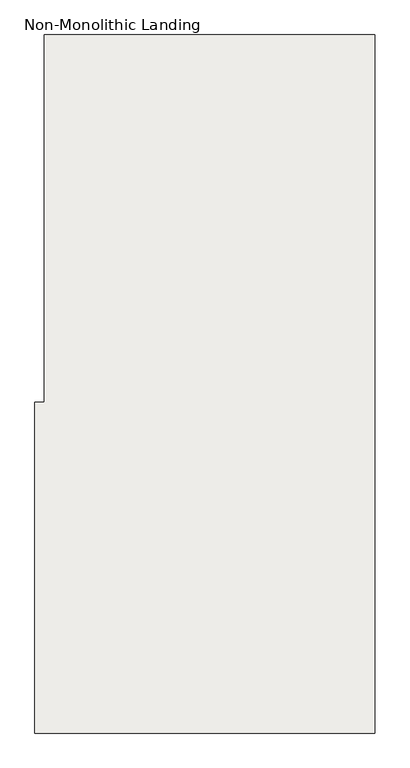
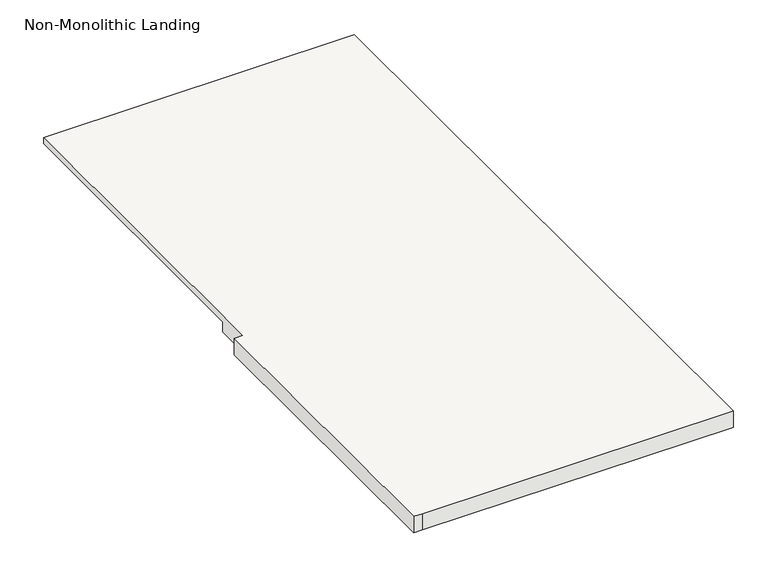
"""IFC4 building model written with IfcOpenShell, lengths in millimetres: slab geometry, Non-Monolithic Landing."""

from ifc_helpers import new_model, si_unit, origin, place, context, project, spatial, faceted_brep, source, transform, mapped, element, save


def non_monolithic_landing_5db28acc(model_context):
    return source(origin(), model_context, "Body", "Brep", [
        faceted_brep([(923.4845537, -3822.9544725, 17583.15), (948.8845537, -3822.9544725, 17557.75), (948.8845537, -4737.3544725, 17557.75), (923.4845537, -4737.3544725, 17583.15), (923.4845537, -4838.9544725, 17602.2), (898.0845537, -4838.9544725, 17602.2), (898.0845537, -5753.3544725, 17602.2), (923.4845537, -5753.3544725, 17602.2), (1837.8845537, -5753.3544725, 17602.2), (1837.8845537, -3822.9544725, 17602.2), (923.4845537, -3822.9544725, 17602.2), (948.8845537, -4737.3544725, 17551.4), (948.8845537, -3822.9544725, 17551.4), (1837.8845537, -3822.9544725, 17551.4), (1837.8845537, -5753.3544725, 17551.4), (923.4845537, -5753.3544725, 17551.4), (898.0845537, -5753.3544725, 17551.4), (898.0845537, -4838.9544725, 17551.4), (923.4845537, -4838.9544725, 17551.4), (923.4845537, -4737.3544725, 17551.4)], [[[0, 1, 2, 3]], [[4, 5, 6, 7, 8, 9, 10]], [[11, 12, 13, 14, 15, 16, 17, 18, 19]], [[12, 11, 2, 1]], [[11, 19, 3, 2]], [[4, 10, 0, 3, 19, 18]], [[5, 4, 18, 17]], [[6, 5, 17, 16]], [[7, 6, 16, 15]], [[8, 7, 15, 14]], [[9, 8, 14, 13]], [[10, 9, 13, 12, 1, 0]]]),
    ])


if __name__ == "__main__":
    model = new_model("IFC4")
    model_context = context("Model", 3, world=origin())
    ifc_project = project(units=[si_unit("LENGTHUNIT", "METRE", prefix="MILLI")], contexts=[model_context])
    site = spatial("IfcSite", under=ifc_project)
    building = spatial("IfcBuilding", under=site)
    placement = place(None, origin())
    non_monolithic_landing_shape = non_monolithic_landing_5db28acc(model_context)
    element("IfcSlab", 1, ObjectType="Non-Monolithic Landing", at=placement, inside=building, context=model_context, shape_type="MappedRepresentation", body=[
        mapped(non_monolithic_landing_shape, transform((0.0, 0.0, 0.0), x_axis=(1.0, 0.0, 0.0), y_axis=(0.0, 1.0, 0.0), z_axis=(0.0, 0.0, 1.0))),
    ])
    save(model, "model.ifc")
